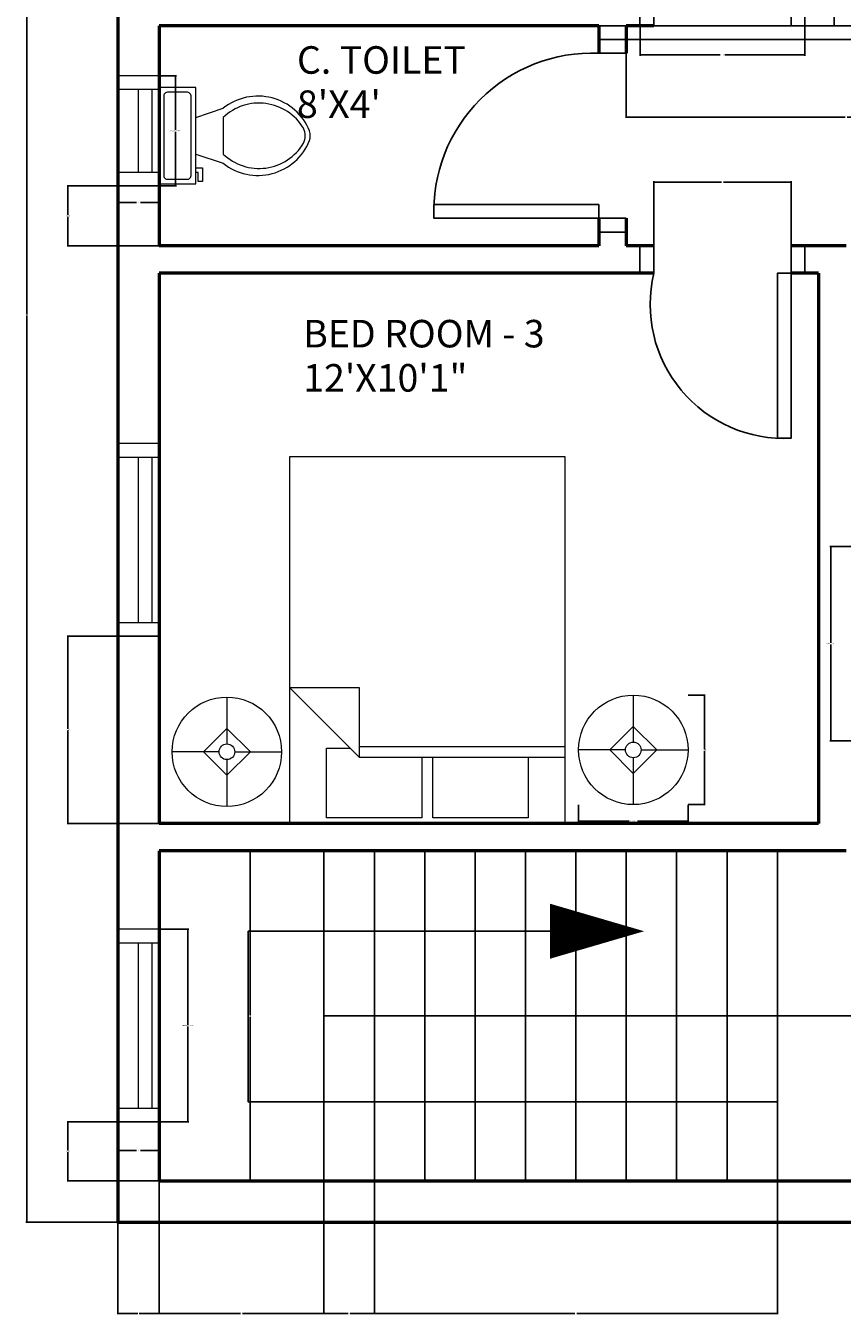
# Model space of a CAD drawing. Units: inches. Extents: x 2630 to 2982, y 643 to 1079.
# Tile 1 of 4: x 2630 to 2808, y 643 to 924. Entities that reach past the tile are written whole.
import ezdxf

# ---------------------------------------------------------------- set-up
doc = ezdxf.new("R2010")
doc.units = ezdxf.units.IN
for name, color, linetype, lineweight in [('A-ANNO-DIMS', 2, 'Continuous', 18), ('A-AREA-IDEN', 7, 'Continuous', 25), ('A-DOOR', 3, 'Continuous', 25), ('A-FLOR-FIXT', 9, 'Continuous', 18), ('A-FLOR-STRS', 7, 'Continuous', 25), ('A-FURN', 8, 'Continuous', 18), ('A-GLAZ', 4, 'Continuous', 18), ('A-WALL', 7, 'Continuous', 50)]:
    doc.layers.add(name, color=color, linetype=linetype, lineweight=lineweight)
doc.styles.get("Standard").update_dxf_attribs({"font": 'arial.ttf'})
doc.dimstyles.get("Standard").update_dxf_attribs({"dimtxt": 0.18, "dimasz": 0.18, "dimexe": 0.18, "dimexo": 0.0625, "dimgap": 0.09, "dimtad": 0, "dimtih": 1, "dimtoh": 1, "dimdec": 4, "dimzin": 0, "dimdsep": 46, "dimtxsty": 'Standard', "dimcen": 0.09, "dimadec": 0, "dimazin": 0, "dimtfac": 1, "dimtdec": 4, "dimtofl": 0, "dimtmove": 0, "dimatfit": 3, "dimfxl": 1, "dimtolj": 1, "dimtzin": 0, "dimarcsym": 0})

# ---------------------------------------------------------------- blocks, each defined once
blk = doc.blocks.new('Bed - Queen')
for p, q in [((0, -80.00003), (0, 0)), ((0, 0), (59.99999, 0)), ((59.99999, 0), (59.99999, -80.00003)), ((7.99999, -1.2), (28.79998, -1.2)), ((7.99999, -14.4), (7.99999, -1.2)), ((28.79998, -1.2), (28.79998, -14.4)), ((31.19999, -1.2), (51.99999, -1.2)), ((31.19999, -14.4), (31.19999, -1.2)), ((51.99999, -1.2), (51.99999, -16.4)), ((0, -14.4), (44.8, -14.4)), ((44.8, -16.8), (0, -16.8)), ((59.99999, -29.6), (44.8, -14.4)), ((44.8, -14.4), (44.8, -29.6)), ((51.99999, -16.4), (46.79936, -16.4)), ((44.8, -29.6), (59.99999, -29.6)), ((59.99999, -80.00003), (0, -80.00003))]:
    blk.add_line(p, q)
blk = doc.blocks.new('Lamp - Table')
for p, q in [((0, 7), (0, 1)), ((0, 3), (-3, 0)), ((3, 0), (0, 3)), ((-1, 0), (-7, 0)), ((-3, 0), (0, -3)), ((0, -3), (3, 0)), ((1, 0), (7, 0)), ((0, -1), (0, -7))]:
    blk.add_line(p, q)
for radius in [7, 1]:
    blk.add_circle((0, 0), radius)
blk = doc.blocks.new('Toilet - top')
for p, q in [((9.5, -6), (9.5, -2)), ((-8, -8.5), (-8, -8)), ((-7, -8), (-7, -9.5)), ((-4, -8), (-6, -14)), ((4, -8), (6, -14)), ((-10, -8.5), (-8, -8.5)), ((-10, -9.5), (-10, -8.5)), ((-7, -9.5), (-10, -9.5)), ((4, -14), (-4, -14))]:
    blk.add_line(p, q)
blk.add_lwpolyline([(10.5, -8), (10.5, 0), (-10.5, 0), (-10.5, -8)], close=True)
for points in [[(-9.5, -2), (-9.5, -6)], [(8.5, -1), (-8.5, -1)], [(-8.5, -7), (8.5, -7)]]:
    blk.add_lwpolyline(points)
for centre, radius, start, end in [((-8.62, -1.88), 0.884, 81.8699, 188.1301), ((8.62, -1.88), 0.884, 351.8699, 98.1301), ((-8.62, -6.12), 0.884, 171.8699, 278.1301), ((8.62, -6.12), 0.884, 261.8699, 8.1301), ((3.52, -21.58), 12.17, 141.4691, 247.9714), ((4.2, -21.82), 11.33, 136.3677, 238.9468), ((-3.52, -21.58), 12.17, 292.0284, 38.5307), ((-4.2, -21.82), 11.33, 301.053, 43.6321), ((0, -27.88), 4, 245.7318, 294.2682), ((0, -29), 4, 254.8605, 285.1395)]:
    blk.add_arc(centre, radius, start, end)
blk = doc.blocks.new('DOOR-30IN-INT')
for p, q in [((0, 6), (0, 0)), ((3, 6), (3, 0)), ((33, 6), (33, 0)), ((36, 6), (36, 0))]:
    blk.add_line(p, q)
blk.add_lwpolyline([(33, 6), (30, 6), (30, 42), (33, 42)], close=True)
blk.add_arc((31.5, 12.75), 29.29, 87.0643, 193.3245)
blk = doc.blocks.new('DOOR-36IN-INT')
for p, q in [((0, 6), (0, 0)), ((3, 6), (3, 0)), ((39, 6), (39, 0)), ((42, 6), (42, 0))]:
    blk.add_line(p, q)
blk.add_lwpolyline([(3, 6), (6, 6), (6, 42), (3, 42)], close=True)
blk.add_arc((4.5, 7.5), 34.53, 357.5104, 92.4896)
blk = doc.blocks.new('WIN-36IN')
for p, q in [((9, 42), (0, 42)), ((9, 39), (0, 39)), ((4.5, 3), (4.5, 39)), ((7.5, 3), (7.5, 39)), ((0, 3), (9, 3)), ((0, 0), (9, 0))]:
    blk.add_line(p, q)
blk = doc.blocks.new('WIN-18IN')
for p, q in [((9, 24), (0, 24)), ((9, 21), (0, 21)), ((1.5, 21), (1.5, 3)), ((4.5, 21), (4.5, 3)), ((0, 3), (9, 3)), ((0, 0), (9, 0))]:
    blk.add_line(p, q)
blk = doc.blocks.new('*D13')
at = {"layer": 'A-ANNO-DIMS', "color": 0, "lineweight": -2, "transparency": 16777216}
for p, q in [((2750.36, 753.89), (2750.36, 750.19)), ((2774.25, 753.89), (2774.25, 750.19)), ((2750.54, 750.37), (2761.41, 750.37)), ((2774.07, 750.37), (2763.21, 750.37))]:
    blk.add_line(p, q, dxfattribs=at)
at = {"layer": 'A-ANNO-DIMS', "color": 0, "transparency": 16777216}
for points in [[(2750.54, 750.4), (2750.54, 750.34), (2750.36, 750.37)], [(2774.07, 750.4), (2774.07, 750.34), (2774.25, 750.37)]]:
    blk.add_solid(points, dxfattribs=at)
at = {"layer": 'Defpoints', "color": 0, "transparency": 16777216}
for p in [(2750.36, 753.95), (2774.25, 753.95), (2774.25, 750.37)]:
    blk.add_point(p, dxfattribs=at)
at = {"layer": 'A-ANNO-DIMS', "color": 0, "transparency": 16777216, "insert": (2762.31, 750.37), "char_height": 0.18, "attachment_point": 5}
blk.add_mtext('\\A1;LAMP 24 TYP.', dxfattribs=at)
blk = doc.blocks.new('*D14')
at = {"layer": 'A-ANNO-DIMS', "color": 0, "lineweight": -2, "transparency": 16777216}
for p, q in [((2774.32, 777.84), (2778.02, 777.84)), ((2777.84, 777.66), (2777.84, 766.08)), ((2777.84, 754.13), (2777.84, 765.72)), ((2774.32, 753.95), (2778.02, 753.95))]:
    blk.add_line(p, q, dxfattribs=at)
at = {"layer": 'A-ANNO-DIMS', "color": 0, "transparency": 16777216}
for points in [[(2777.81, 777.66), (2777.87, 777.66), (2777.84, 777.84)], [(2777.81, 754.13), (2777.87, 754.13), (2777.84, 753.95)]]:
    blk.add_solid(points, dxfattribs=at)
at = {"layer": 'Defpoints', "color": 0, "transparency": 16777216}
for p in [(2774.25, 777.84), (2777.84, 777.84), (2774.25, 753.95)]:
    blk.add_point(p, dxfattribs=at)
at = {"layer": 'A-ANNO-DIMS', "color": 0, "transparency": 16777216, "insert": (2777.84, 765.9), "char_height": 0.18, "attachment_point": 5}
blk.add_mtext('\\A1;24 TYP.', dxfattribs=at)
blk = doc.blocks.new('*D15')
at = {"layer": 'A-ANNO-DIMS', "color": 0, "lineweight": -2, "transparency": 16777216}
for p, q in [((2658.83, 726.76), (2665.25, 726.76)), ((2665.07, 726.58), (2665.07, 705.94)), ((2665.07, 684.94), (2665.07, 705.58)), ((2658.83, 684.76), (2665.25, 684.76))]:
    blk.add_line(p, q, dxfattribs=at)
at = {"layer": 'A-ANNO-DIMS', "color": 0, "transparency": 16777216}
for points in [[(2665.04, 726.58), (2665.1, 726.58), (2665.07, 726.76)], [(2665.04, 684.94), (2665.1, 684.94), (2665.07, 684.76)]]:
    blk.add_solid(points, dxfattribs=at)
at = {"layer": 'Defpoints', "color": 0, "transparency": 16777216}
for p in [(2658.77, 726.76), (2665.07, 726.76), (2658.77, 684.76)]:
    blk.add_point(p, dxfattribs=at)
at = {"layer": 'A-ANNO-DIMS', "color": 0, "transparency": 16777216, "insert": (2665.07, 705.76), "char_height": 0.18, "attachment_point": 5}
blk.add_mtext('\\A1;WINDOW W1 42 TYP.', dxfattribs=at)
blk = doc.blocks.new('*D16')
at = {"layer": 'A-ANNO-DIMS', "color": 0, "lineweight": -2, "transparency": 16777216}
for p, q in [((2649.77, 684.7), (2649.77, 678.28)), ((2658.77, 684.7), (2658.77, 678.28)), ((2649.95, 678.46), (2653.81, 678.46)), ((2658.59, 678.46), (2654.73, 678.46))]:
    blk.add_line(p, q, dxfattribs=at)
at = {"layer": 'A-ANNO-DIMS', "color": 0, "transparency": 16777216}
for points in [[(2649.95, 678.49), (2649.95, 678.43), (2649.77, 678.46)], [(2658.59, 678.49), (2658.59, 678.43), (2658.77, 678.46)]]:
    blk.add_solid(points, dxfattribs=at)
at = {"layer": 'Defpoints', "color": 0, "transparency": 16777216}
for p in [(2649.77, 684.76), (2658.77, 684.76), (2658.77, 678.46)]:
    blk.add_point(p, dxfattribs=at)
at = {"layer": 'A-ANNO-DIMS', "color": 0, "transparency": 16777216, "insert": (2654.27, 678.46), "char_height": 0.18, "attachment_point": 5}
blk.add_mtext('\\A1;9 TYP.', dxfattribs=at)
blk = doc.blocks.new('*D19')
at = {"layer": 'A-ANNO-DIMS', "color": 0, "lineweight": -2, "transparency": 16777216}
for p, q in [((2811.7, 810.29), (2805.22, 810.29)), ((2805.4, 810.11), (2805.4, 789.26)), ((2805.4, 768.05), (2805.4, 788.89)), ((2811.7, 767.87), (2805.22, 767.87))]:
    blk.add_line(p, q, dxfattribs=at)
at = {"layer": 'A-ANNO-DIMS', "color": 0, "transparency": 16777216}
for points in [[(2805.37, 810.11), (2805.43, 810.11), (2805.4, 810.29)], [(2805.37, 768.05), (2805.43, 768.05), (2805.4, 767.87)]]:
    blk.add_solid(points, dxfattribs=at)
at = {"layer": 'Defpoints', "color": 0, "transparency": 16777216}
for p in [(2805.4, 810.29), (2811.77, 810.29), (2811.77, 767.87)]:
    blk.add_point(p, dxfattribs=at)
at = {"layer": 'A-ANNO-DIMS', "color": 0, "transparency": 16777216, "insert": (2805.4, 789.08), "char_height": 0.18, "attachment_point": 5}
blk.add_mtext('\\A1;DOOR D1 42 TYP.', dxfattribs=at)
blk = doc.blocks.new('*D25')
at = {"layer": 'A-ANNO-DIMS', "color": 0, "lineweight": -2, "transparency": 16777216}
for p, q in [((2799.83, 966.34), (2806.32, 966.34)), ((2806.14, 966.16), (2806.14, 945.29)), ((2806.14, 924.05), (2806.14, 944.92)), ((2799.83, 923.87), (2806.32, 923.87))]:
    blk.add_line(p, q, dxfattribs=at)
at = {"layer": 'A-ANNO-DIMS', "color": 0, "transparency": 16777216}
for points in [[(2806.11, 966.16), (2806.17, 966.16), (2806.14, 966.34)], [(2806.11, 924.05), (2806.17, 924.05), (2806.14, 923.87)]]:
    blk.add_solid(points, dxfattribs=at)
at = {"layer": 'Defpoints', "color": 0, "transparency": 16777216}
for p in [(2799.77, 966.34), (2806.14, 966.34), (2799.77, 923.87)]:
    blk.add_point(p, dxfattribs=at)
at = {"layer": 'A-ANNO-DIMS', "color": 0, "transparency": 16777216, "insert": (2806.14, 945.1), "char_height": 0.18, "attachment_point": 5}
blk.add_mtext('\\A1;DOOR D2 42 TYP.', dxfattribs=at)
blk = doc.blocks.new('*D26')
at = {"layer": 'A-ANNO-DIMS', "color": 0, "lineweight": -2, "transparency": 16777216}
for p, q in [((2763.77, 923.8), (2763.77, 917.32)), ((2799.77, 923.8), (2799.77, 917.32)), ((2763.95, 917.5), (2781.24, 917.5)), ((2799.59, 917.5), (2782.3, 917.5))]:
    blk.add_line(p, q, dxfattribs=at)
at = {"layer": 'A-ANNO-DIMS', "color": 0, "transparency": 16777216}
for points in [[(2763.95, 917.53), (2763.95, 917.47), (2763.77, 917.5)], [(2799.59, 917.53), (2799.59, 917.47), (2799.77, 917.5)]]:
    blk.add_solid(points, dxfattribs=at)
at = {"layer": 'Defpoints', "color": 0, "transparency": 16777216}
for p in [(2763.77, 923.87), (2799.77, 923.87), (2799.77, 917.5)]:
    blk.add_point(p, dxfattribs=at)
at = {"layer": 'A-ANNO-DIMS', "color": 0, "transparency": 16777216, "insert": (2781.77, 917.5), "char_height": 0.18, "attachment_point": 5}
blk.add_mtext('\\A1;36 TYP.', dxfattribs=at)
blk = doc.blocks.new('*D27')
at = {"layer": 'A-ANNO-DIMS', "color": 0, "lineweight": -2, "transparency": 16777216}
for p, q in [((2658.83, 912.94), (2662.55, 912.94)), ((2662.37, 912.76), (2662.37, 901.13)), ((2662.37, 889.12), (2662.37, 900.76)), ((2658.83, 888.94), (2662.55, 888.94))]:
    blk.add_line(p, q, dxfattribs=at)
at = {"layer": 'A-ANNO-DIMS', "color": 0, "transparency": 16777216}
for points in [[(2662.34, 912.76), (2662.4, 912.76), (2662.37, 912.94)], [(2662.34, 889.12), (2662.4, 889.12), (2662.37, 888.94)]]:
    blk.add_solid(points, dxfattribs=at)
at = {"layer": 'Defpoints', "color": 0, "transparency": 16777216}
for p in [(2658.77, 912.94), (2658.77, 888.94), (2662.37, 888.94)]:
    blk.add_point(p, dxfattribs=at)
at = {"layer": 'A-ANNO-DIMS', "color": 0, "transparency": 16777216, "insert": (2662.37, 900.94), "char_height": 0.18, "attachment_point": 5}
blk.add_mtext('\\A1;WINDOW W2 24 TYP.', dxfattribs=at)
blk = doc.blocks.new('*D28')
at = {"layer": 'A-ANNO-DIMS', "color": 0, "lineweight": -2, "transparency": 16777216}
for p, q in [((2649.77, 888.88), (2649.77, 885.16)), ((2658.77, 888.88), (2658.77, 885.16)), ((2649.95, 885.34), (2653.81, 885.34)), ((2658.59, 885.34), (2654.73, 885.34))]:
    blk.add_line(p, q, dxfattribs=at)
at = {"layer": 'A-ANNO-DIMS', "color": 0, "transparency": 16777216}
for points in [[(2649.95, 885.37), (2649.95, 885.31), (2649.77, 885.34)], [(2658.59, 885.37), (2658.59, 885.31), (2658.77, 885.34)]]:
    blk.add_solid(points, dxfattribs=at)
at = {"layer": 'Defpoints', "color": 0, "transparency": 16777216}
for p in [(2649.77, 888.94), (2658.77, 888.94), (2649.77, 885.34)]:
    blk.add_point(p, dxfattribs=at)
at = {"layer": 'A-ANNO-DIMS', "color": 0, "transparency": 16777216, "insert": (2654.27, 885.34), "char_height": 0.18, "attachment_point": 5}
blk.add_mtext('\\A1;9 TYP.', dxfattribs=at)
blk = doc.blocks.new('*D38')
at = {"layer": 'A-ANNO-DIMS', "color": 0, "lineweight": -2, "transparency": 16777216}
for p, q in [((2649.7, 1058.87), (2629.68, 1058.87)), ((2629.86, 1058.69), (2629.86, 861.05)), ((2629.86, 663.05), (2629.86, 860.68)), ((2649.7, 662.87), (2629.68, 662.87))]:
    blk.add_line(p, q, dxfattribs=at)
at = {"layer": 'A-ANNO-DIMS', "color": 0, "transparency": 16777216}
for points in [[(2629.83, 1058.69), (2629.89, 1058.69), (2629.86, 1058.87)], [(2629.83, 663.05), (2629.89, 663.05), (2629.86, 662.87)]]:
    blk.add_solid(points, dxfattribs=at)
at = {"layer": 'Defpoints', "color": 0, "transparency": 16777216}
for p in [(2629.86, 1058.87), (2649.77, 1058.87), (2649.77, 662.87)]:
    blk.add_point(p, dxfattribs=at)
at = {"layer": 'A-ANNO-DIMS', "color": 0, "transparency": 16777216, "insert": (2629.86, 860.87), "char_height": 0.18, "attachment_point": 5}
blk.add_mtext('\\A1;396', dxfattribs=at)
blk = doc.blocks.new('*D39')
at = {"layer": 'A-ANNO-DIMS', "color": 0, "lineweight": -2, "transparency": 16777216}
for p, q in [((2658.77, 671.8), (2658.77, 642.78)), ((2649.77, 662.8), (2649.77, 642.78)), ((2649.95, 642.96), (2654.12, 642.96)), ((2658.59, 642.96), (2654.42, 642.96))]:
    blk.add_line(p, q, dxfattribs=at)
at = {"layer": 'A-ANNO-DIMS', "color": 0, "transparency": 16777216}
for points in [[(2649.95, 642.99), (2649.95, 642.93), (2649.77, 642.96)], [(2658.59, 642.99), (2658.59, 642.93), (2658.77, 642.96)]]:
    blk.add_solid(points, dxfattribs=at)
at = {"layer": 'Defpoints', "color": 0, "transparency": 16777216}
for p in [(2658.77, 671.87), (2649.77, 662.87), (2658.77, 642.96)]:
    blk.add_point(p, dxfattribs=at)
at = {"layer": 'A-ANNO-DIMS', "color": 0, "transparency": 16777216, "insert": (2654.27, 642.96), "char_height": 0.18, "attachment_point": 5}
blk.add_mtext('\\A1;9', dxfattribs=at)
blk = doc.blocks.new('*D42')
at = {"layer": 'A-ANNO-DIMS', "color": 0, "lineweight": -2, "transparency": 16777216}
for p, q in [((2658.7, 888.94), (2638.68, 888.94)), ((2638.86, 888.76), (2638.86, 882.59)), ((2638.86, 876.05), (2638.86, 882.22)), ((2658.7, 875.87), (2638.68, 875.87))]:
    blk.add_line(p, q, dxfattribs=at)
at = {"layer": 'A-ANNO-DIMS', "color": 0, "transparency": 16777216}
for points in [[(2638.83, 888.76), (2638.89, 888.76), (2638.86, 888.94)], [(2638.83, 876.05), (2638.89, 876.05), (2638.86, 875.87)]]:
    blk.add_solid(points, dxfattribs=at)
at = {"layer": 'Defpoints', "color": 0, "transparency": 16777216}
for p in [(2638.86, 888.94), (2658.77, 888.94), (2658.77, 875.87)]:
    blk.add_point(p, dxfattribs=at)
at = {"layer": 'A-ANNO-DIMS', "color": 0, "transparency": 16777216, "insert": (2638.86, 882.41), "char_height": 0.18, "attachment_point": 5}
blk.add_mtext('\\A1;13.078', dxfattribs=at)
blk = doc.blocks.new('*D43')
at = {"layer": 'A-ANNO-DIMS', "color": 0, "lineweight": -2, "transparency": 16777216}
for p, q in [((2658.7, 790.7), (2638.68, 790.7)), ((2638.86, 790.52), (2638.86, 770.47)), ((2638.86, 750.05), (2638.86, 770.1)), ((2658.7, 749.87), (2638.68, 749.87))]:
    blk.add_line(p, q, dxfattribs=at)
at = {"layer": 'A-ANNO-DIMS', "color": 0, "transparency": 16777216}
for points in [[(2638.83, 790.52), (2638.89, 790.52), (2638.86, 790.7)], [(2638.83, 750.05), (2638.89, 750.05), (2638.86, 749.87)]]:
    blk.add_solid(points, dxfattribs=at)
at = {"layer": 'Defpoints', "color": 0, "transparency": 16777216}
for p in [(2638.86, 790.7), (2658.77, 790.7), (2658.77, 749.87)]:
    blk.add_point(p, dxfattribs=at)
at = {"layer": 'A-ANNO-DIMS', "color": 0, "transparency": 16777216, "insert": (2638.86, 770.28), "char_height": 0.18, "attachment_point": 5}
blk.add_mtext('\\A1;40.83', dxfattribs=at)
blk = doc.blocks.new('*D44')
at = {"layer": 'A-ANNO-DIMS', "color": 0, "lineweight": -2, "transparency": 16777216}
for p, q in [((2658.7, 684.76), (2638.68, 684.76)), ((2638.86, 684.58), (2638.86, 678.5)), ((2638.86, 672.05), (2638.86, 678.13)), ((2658.7, 671.87), (2638.68, 671.87))]:
    blk.add_line(p, q, dxfattribs=at)
at = {"layer": 'A-ANNO-DIMS', "color": 0, "transparency": 16777216}
for points in [[(2638.83, 684.58), (2638.89, 684.58), (2638.86, 684.76)], [(2638.83, 672.05), (2638.89, 672.05), (2638.86, 671.87)]]:
    blk.add_solid(points, dxfattribs=at)
at = {"layer": 'Defpoints', "color": 0, "transparency": 16777216}
for p in [(2638.86, 684.76), (2658.77, 684.76), (2658.77, 671.87)]:
    blk.add_point(p, dxfattribs=at)
at = {"layer": 'A-ANNO-DIMS', "color": 0, "transparency": 16777216, "insert": (2638.86, 678.31), "char_height": 0.18, "attachment_point": 5}
blk.add_mtext('\\A1;12.894', dxfattribs=at)
blk = doc.blocks.new('*D53')
at = {"layer": 'A-ANNO-DIMS', "color": 0, "lineweight": -2, "transparency": 16777216}
for p, q in [((2793.83, 707.87), (2813.86, 707.87)), ((2813.68, 707.69), (2813.68, 690.05)), ((2813.68, 672.05), (2813.68, 689.68)), ((2793.83, 671.87), (2813.86, 671.87))]:
    blk.add_line(p, q, dxfattribs=at)
at = {"layer": 'A-ANNO-DIMS', "color": 0, "transparency": 16777216}
for points in [[(2813.65, 707.69), (2813.71, 707.69), (2813.68, 707.87)], [(2813.65, 672.05), (2813.71, 672.05), (2813.68, 671.87)]]:
    blk.add_solid(points, dxfattribs=at)
at = {"layer": 'Defpoints', "color": 0, "transparency": 16777216}
for p in [(2793.77, 707.87), (2793.77, 671.87), (2813.68, 671.87)]:
    blk.add_point(p, dxfattribs=at)
at = {"layer": 'A-ANNO-DIMS', "color": 0, "transparency": 16777216, "insert": (2813.68, 689.87), "char_height": 0.18, "attachment_point": 5}
blk.add_mtext('\\A1;36', dxfattribs=at)
blk = doc.blocks.new('*D54')
at = {"layer": 'A-ANNO-DIMS', "color": 0, "lineweight": -2, "transparency": 16777216}
for p, q in [((2658.77, 671.8), (2658.77, 642.78)), ((2694.77, 671.8), (2694.77, 642.78)), ((2658.95, 642.96), (2676.55, 642.96)), ((2694.59, 642.96), (2676.99, 642.96))]:
    blk.add_line(p, q, dxfattribs=at)
at = {"layer": 'A-ANNO-DIMS', "color": 0, "transparency": 16777216}
for points in [[(2658.95, 642.99), (2658.95, 642.93), (2658.77, 642.96)], [(2694.59, 642.99), (2694.59, 642.93), (2694.77, 642.96)]]:
    blk.add_solid(points, dxfattribs=at)
at = {"layer": 'Defpoints', "color": 0, "transparency": 16777216}
for p in [(2658.77, 671.87), (2694.77, 671.87), (2694.77, 642.96)]:
    blk.add_point(p, dxfattribs=at)
at = {"layer": 'A-ANNO-DIMS', "color": 0, "transparency": 16777216, "insert": (2676.77, 642.96), "char_height": 0.18, "attachment_point": 5}
blk.add_mtext('\\A1;36', dxfattribs=at)
blk = doc.blocks.new('*D55')
at = {"layer": 'A-ANNO-DIMS', "color": 0, "lineweight": -2, "transparency": 16777216}
for p, q in [((2694.77, 671.8), (2694.77, 642.78)), ((2705.77, 671.8), (2705.77, 642.78)), ((2694.95, 642.96), (2700.07, 642.96)), ((2705.59, 642.96), (2700.46, 642.96))]:
    blk.add_line(p, q, dxfattribs=at)
at = {"layer": 'A-ANNO-DIMS', "color": 0, "transparency": 16777216}
for points in [[(2694.95, 642.99), (2694.95, 642.93), (2694.77, 642.96)], [(2705.59, 642.99), (2705.59, 642.93), (2705.77, 642.96)]]:
    blk.add_solid(points, dxfattribs=at)
at = {"layer": 'Defpoints', "color": 0, "transparency": 16777216}
for p in [(2694.77, 671.87), (2705.77, 671.87), (2705.77, 642.96)]:
    blk.add_point(p, dxfattribs=at)
at = {"layer": 'A-ANNO-DIMS', "color": 0, "transparency": 16777216, "insert": (2700.27, 642.96), "char_height": 0.18, "attachment_point": 5}
blk.add_mtext('\\A1;11', dxfattribs=at)
blk = doc.blocks.new('*D56')
at = {"layer": 'A-ANNO-DIMS', "color": 0, "lineweight": -2, "transparency": 16777216}
for p, q in [((2705.77, 671.8), (2705.77, 642.78)), ((2793.77, 671.8), (2793.77, 642.78)), ((2705.95, 642.96), (2749.55, 642.96)), ((2793.59, 642.96), (2749.99, 642.96))]:
    blk.add_line(p, q, dxfattribs=at)
at = {"layer": 'A-ANNO-DIMS', "color": 0, "transparency": 16777216}
for points in [[(2705.95, 642.99), (2705.95, 642.93), (2705.77, 642.96)], [(2793.59, 642.99), (2793.59, 642.93), (2793.77, 642.96)]]:
    blk.add_solid(points, dxfattribs=at)
at = {"layer": 'Defpoints', "color": 0, "transparency": 16777216}
for p in [(2705.77, 671.87), (2793.77, 671.87), (2793.77, 642.96)]:
    blk.add_point(p, dxfattribs=at)
at = {"layer": 'A-ANNO-DIMS', "color": 0, "transparency": 16777216, "insert": (2749.77, 642.96), "char_height": 0.18, "attachment_point": 5}
blk.add_mtext('\\A1;88', dxfattribs=at)
blk = doc.blocks.new('*D61')
at = {"layer": 'A-ANNO-DIMS', "color": 0, "lineweight": -2, "transparency": 16777216}
for p, q in [((2754.83, 923.87), (2981.86, 923.87)), ((2981.68, 923.69), (2981.68, 922.55)), ((2981.68, 921.05), (2981.68, 922.18)), ((2754.83, 920.87), (2981.86, 920.87))]:
    blk.add_line(p, q, dxfattribs=at)
at = {"layer": 'A-ANNO-DIMS', "color": 0, "transparency": 16777216}
for points in [[(2981.65, 923.69), (2981.71, 923.69), (2981.68, 923.87)], [(2981.65, 921.05), (2981.71, 921.05), (2981.68, 920.87)]]:
    blk.add_solid(points, dxfattribs=at)
at = {"layer": 'Defpoints', "color": 0, "transparency": 16777216}
for p in [(2754.77, 923.87), (2754.77, 920.87), (2981.68, 920.87)]:
    blk.add_point(p, dxfattribs=at)
at = {"layer": 'A-ANNO-DIMS', "color": 0, "transparency": 16777216, "insert": (2981.68, 922.37), "char_height": 0.18, "attachment_point": 5}
blk.add_mtext('\\A1;3', dxfattribs=at)
blk = doc.blocks.new('*D62')
at = {"layer": 'A-ANNO-DIMS', "color": 0, "lineweight": -2, "transparency": 16777216}
for p, q in [((2766.77, 869.93), (2766.77, 889.96)), ((2766.95, 889.78), (2781.55, 889.78)), ((2796.59, 889.78), (2781.99, 889.78)), ((2796.77, 869.93), (2796.77, 889.96))]:
    blk.add_line(p, q, dxfattribs=at)
at = {"layer": 'A-ANNO-DIMS', "color": 0, "transparency": 16777216}
for points in [[(2766.95, 889.81), (2766.95, 889.75), (2766.77, 889.78)], [(2796.59, 889.81), (2796.59, 889.75), (2796.77, 889.78)]]:
    blk.add_solid(points, dxfattribs=at)
at = {"layer": 'Defpoints', "color": 0, "transparency": 16777216}
for p in [(2796.77, 889.78), (2766.77, 869.87), (2796.77, 869.87)]:
    blk.add_point(p, dxfattribs=at)
at = {"layer": 'A-ANNO-DIMS', "color": 0, "transparency": 16777216, "insert": (2781.77, 889.78), "char_height": 0.18, "attachment_point": 5}
blk.add_mtext('\\A1;30', dxfattribs=at)
blk = doc.blocks.new('*D64')
at = {"layer": 'A-ANNO-DIMS', "color": 0, "lineweight": -2, "transparency": 16777216}
for p, q in [((2760.77, 923.8), (2760.77, 903.78)), ((2856.77, 923.8), (2856.77, 903.78)), ((2760.95, 903.96), (2808.55, 903.96)), ((2856.59, 903.96), (2808.99, 903.96))]:
    blk.add_line(p, q, dxfattribs=at)
at = {"layer": 'A-ANNO-DIMS', "color": 0, "transparency": 16777216}
for points in [[(2760.95, 903.99), (2760.95, 903.93), (2760.77, 903.96)], [(2856.59, 903.99), (2856.59, 903.93), (2856.77, 903.96)]]:
    blk.add_solid(points, dxfattribs=at)
at = {"layer": 'Defpoints', "color": 0, "transparency": 16777216}
for p in [(2760.77, 923.87), (2856.77, 923.87), (2760.77, 903.96)]:
    blk.add_point(p, dxfattribs=at)
at = {"layer": 'A-ANNO-DIMS', "color": 0, "transparency": 16777216, "insert": (2808.77, 903.96), "char_height": 0.18, "attachment_point": 5}
blk.add_mtext('\\A1;96', dxfattribs=at)
blk = doc.blocks.new('*D65')
at = {"layer": 'A-ANNO-DIMS', "color": 0, "lineweight": -2, "transparency": 16777216}
for p, q in [((2658.83, 743.87), (2678.86, 743.87)), ((2678.68, 743.69), (2678.68, 708.05)), ((2678.68, 672.05), (2678.68, 707.69)), ((2658.83, 671.87), (2678.86, 671.87))]:
    blk.add_line(p, q, dxfattribs=at)
at = {"layer": 'A-ANNO-DIMS', "color": 0, "transparency": 16777216}
for points in [[(2678.65, 743.69), (2678.71, 743.69), (2678.68, 743.87)], [(2678.65, 672.05), (2678.71, 672.05), (2678.68, 671.87)]]:
    blk.add_solid(points, dxfattribs=at)
at = {"layer": 'Defpoints', "color": 0, "transparency": 16777216}
for p in [(2658.77, 743.87), (2658.77, 671.87), (2678.68, 671.87)]:
    blk.add_point(p, dxfattribs=at)
at = {"layer": 'A-ANNO-DIMS', "color": 0, "transparency": 16777216, "insert": (2678.68, 707.87), "char_height": 0.18, "attachment_point": 5}
blk.add_mtext('\\A1;72', dxfattribs=at)

msp = doc.modelspace()

# ---------------------------------------------------------------- linework, layer by layer
at = {"layer": 'A-FLOR-STRS'}
for p, q in [((2694.7671, 743.8666), (2694.7671, 671.8666)), ((2705.7671, 743.8666), (2705.7671, 671.8666)), ((2716.7671, 743.8666), (2716.7671, 671.8666)), ((2727.7671, 743.8666), (2727.7671, 671.8666)), ((2738.7671, 743.8666), (2738.7671, 671.8666)), ((2749.7671, 743.8666), (2749.7671, 671.8666)), ((2760.7671, 743.8666), (2760.7671, 671.8666)), ((2771.7671, 743.8666), (2771.7671, 671.8666)), ((2782.7671, 743.8666), (2782.7671, 671.8666)), ((2793.7671, 743.8666), (2793.7671, 671.8666)), ((2793.7671, 707.8666), (2694.7671, 707.8666))]:
    msp.add_line(p, q, dxfattribs=at)
msp.add_lwpolyline([(2744.1329, 726.3329, 12, 0, 0), (2764.6647, 726.3329, 0, 0, 0)], format="xyseb", dxfattribs=at)
msp.add_lwpolyline([(2793.7671, 689.0821), (2678.2153, 689.0821), (2678.2153, 726.3329), (2744.1329, 726.3329)], dxfattribs=at)
at = {"layer": 'A-WALL'}
for p, q in [((2658.7671, 923.8666), (2658.7671, 875.8666)), ((2754.7671, 923.8666), (2658.7671, 923.8666)), ((2754.7671, 923.8666), (2754.7671, 917.8666)), ((2760.7671, 923.8666), (2760.7671, 917.8666)), ((2766.7671, 923.8666), (2760.7671, 923.8666)), ((2754.7671, 881.8666), (2754.7671, 875.8666)), ((2760.7671, 881.8666), (2760.7671, 875.8666)), ((2754.7671, 875.8666), (2658.7671, 875.8666)), ((2766.7671, 875.8666), (2760.7671, 875.8666)), ((2808.7671, 875.8666), (2796.7671, 875.8666)), ((2658.7671, 869.8666), (2658.7671, 749.8666)), ((2766.7671, 869.8666), (2658.7671, 869.8666)), ((2802.7671, 869.8666), (2796.7671, 869.8666)), ((2802.7671, 869.8666), (2802.7671, 749.8666)), ((2802.7671, 749.8666), (2658.7671, 749.8666)), ((2808.7671, 743.8666), (2658.7671, 743.8666)), ((2658.7671, 743.8666), (2658.7671, 671.8666)), ((2658.7671, 671.8666), (2814.7671, 671.8666))]:
    msp.add_line(p, q, dxfattribs=at)
msp.add_lwpolyline([(2850.7671, 662.8666), (2961.7671, 662.8666), (2961.7671, 1058.8666), (2649.7671, 1058.8666), (2649.7671, 662.8666), (2814.7671, 662.8666)], dxfattribs=at)

# ---------------------------------------------------------------- block references
at = {"layer": 'A-DOOR'}
msp.add_blockref('DOOR-30IN-INT', (2763.767, 923.867), dxfattribs=at)
at = {"layer": 'A-DOOR', "rotation": 90.00000000000036}
msp.add_blockref('DOOR-36IN-INT', (2760.7667, 878.8665), dxfattribs=at)
at = {"layer": 'A-DOOR', "extrusion": (0, 0, -1), "zscale": -1, "rotation": 180}
msp.add_blockref('DOOR-30IN-INT', (-2763.767, 875.8663), dxfattribs=at)
at = {"layer": 'A-FLOR-FIXT', "rotation": 90}
msp.add_blockref('Toilet - top', (2658.7671, 899.8666), dxfattribs=at)
at = {"layer": 'A-FURN', "rotation": 180}
msp.add_blockref('Bed - Queen', (2747.3366, 749.8666), dxfattribs=at)
at = {"layer": 'A-FURN', "xscale": 1.706595897520738, "yscale": 1.706595897520738, "zscale": 1.706595897520738}
for p in [(2673.5711, 765.4739), (2762.3072, 765.8961)]:
    msp.add_blockref('Lamp - Table', p, dxfattribs=at)
at = {"layer": 'A-GLAZ', "rotation": 180}
msp.add_blockref('WIN-18IN', (2658.7672, 912.9445), dxfattribs=at)
at = {"layer": 'A-GLAZ'}
for p in [(2649.767, 790.6998), (2649.767, 684.7608)]:
    msp.add_blockref('WIN-36IN', p, dxfattribs=at)

# ---------------------------------------------------------------- texts
at = {"layer": 'A-AREA-IDEN'}
for s, p in [('C. TOILET', (2688.8661, 913.4037)), ("8'X4'", (2688.8661, 903.7653)), ('BED ROOM - 3', (2690.233, 853.6959)), ('12\'X10\'1"', (2690.233, 844.0574))]:
    msp.add_text(s, height=6, dxfattribs=at).set_placement(p)

# ---------------------------------------------------------------- dimensions: what is measured, and where the dimension line sits
at = {"layer": 'A-ANNO-DIMS'}
for base, p1, p2, angle, override, picture, middle in [((2629.8571, 1058.8666), (2649.7671, 662.8666), (2649.7671, 1058.8666), 90, {"dimdec": 0, "dimlfac": 1, "dimrnd": 0, "dimzin": 0, "dimdsep": 46, "dimlunit": 2}, '*D38', (2629.8571, 860.8666)), ((2981.6771, 920.8666), (2754.7671, 923.8666), (2754.7671, 920.8666), 90, {"dimdec": 0, "dimlfac": 1, "dimrnd": 0, "dimzin": 0, "dimdsep": 46, "dimlunit": 2}, '*D61', (2981.6771, 922.3666)), ((2760.7671, 903.9566), (2856.7671, 923.8666), (2760.7671, 923.8666), 180, {"dimdec": 0, "dimlfac": 1, "dimrnd": 0, "dimzin": 0, "dimdsep": 46, "dimlunit": 2}, '*D64', (2808.7671, 903.9566)), ((2638.8571, 888.9447), (2658.7671, 875.8666), (2658.7671, 888.9447), 90, {"dimdec": 3, "dimlfac": 1, "dimrnd": 0, "dimzin": 0, "dimdsep": 46, "dimlunit": 2}, '*D42', (2638.8571, 882.4057)), ((2638.8571, 790.6997), (2658.7671, 749.8666), (2658.7671, 790.6997), 90, {"dimdec": 2, "dimlfac": 1, "dimrnd": 0, "dimzin": 0, "dimdsep": 46, "dimlunit": 2}, '*D43', (2638.8571, 770.2832)), ((2678.6771, 671.8666), (2658.7671, 743.8666), (2658.7671, 671.8666), 270, {"dimdec": 0, "dimlfac": 1, "dimrnd": 0, "dimzin": 0, "dimdsep": 46, "dimlunit": 2}, '*D65', (2678.6771, 707.8666)), ((2813.6771, 671.8666), (2793.7671, 707.8666), (2793.7671, 671.8666), 270, {"dimdec": 0, "dimlfac": 1, "dimrnd": 0, "dimzin": 0, "dimdsep": 46, "dimlunit": 2}, '*D53', (2813.6771, 689.8666)), ((2638.8571, 684.7607), (2658.7671, 671.8666), (2658.7671, 684.7607), 90, {"dimdec": 3, "dimlfac": 1, "dimrnd": 0, "dimzin": 0, "dimdsep": 46, "dimlunit": 2}, '*D44', (2638.8571, 678.3137))]:
    dim = msp.add_linear_dim(base=base, p1=p1, p2=p2, angle=angle, dimstyle='Standard', override=override, dxfattribs=at)
    dim.commit()
    dim.dimension.update_dxf_attribs({"geometry": picture, "text_midpoint": middle})
for base, p1, p2, angle, text, picture, middle in [((2806.1379, 966.3388), (2799.7671, 923.8666), (2799.7671, 966.3388), 90, 'DOOR D2 <> TYP.', '*D25', (2806.1379, 945.1027)), ((2662.3671, 888.9447), (2658.7671, 912.9447), (2658.7671, 888.9447), 270, 'WINDOW W2 <> TYP.', '*D27', (2662.3671, 900.9447)), ((2649.7671, 885.3447), (2658.7671, 888.9447), (2649.7671, 888.9447), 180, '<> TYP.', '*D28', (2654.2671, 885.3447)), ((2805.404, 810.2871), (2811.7671, 767.8666), (2811.7671, 810.2871), 90, 'DOOR D1 <> TYP.', '*D19', (2805.404, 789.0769)), ((2777.8372, 777.8423), (2774.2534, 753.9499), (2774.2534, 777.8423), 90, '<> TYP.', '*D14', (2777.8372, 765.8961)), ((2665.0671, 726.7607), (2658.7671, 684.7607), (2658.7671, 726.7607), 90, 'WINDOW W1 <> TYP.', '*D15', (2665.0671, 705.7607))]:
    dim = msp.add_linear_dim(base=base, p1=p1, p2=p2, angle=angle, text=text, dimstyle='Standard', override={"dimdec": 0, "dimlfac": 1, "dimrnd": 0, "dimzin": 0, "dimdsep": 46, "dimlunit": 2}, dxfattribs=at)
    dim.commit()
    dim.dimension.update_dxf_attribs({"geometry": picture, "text_midpoint": middle})
for base, p1, p2, text, picture, middle in [((2799.7671, 917.4958), (2763.7671, 923.8666), (2799.7671, 923.8666), '<> TYP.', '*D26', (2781.7671, 917.4958)), ((2774.2534, 750.3661), (2750.361, 753.9499), (2774.2534, 753.9499), 'LAMP <> TYP.', '*D13', (2762.3072, 750.3661)), ((2658.7671, 678.4607), (2649.7671, 684.7607), (2658.7671, 684.7607), '<> TYP.', '*D16', (2654.2671, 678.4607))]:
    dim = msp.add_linear_dim(base=base, p1=p1, p2=p2, text=text, dimstyle='Standard', override={"dimdec": 0, "dimlfac": 1, "dimrnd": 0, "dimzin": 0, "dimdsep": 46, "dimlunit": 2}, dxfattribs=at)
    dim.commit()
    dim.dimension.update_dxf_attribs({"geometry": picture, "text_midpoint": middle})
for base, p1, p2, picture, middle in [((2796.7671, 889.7766), (2766.7671, 869.8666), (2796.7671, 869.8666), '*D62', (2781.7671, 889.7766)), ((2658.7671, 642.9566), (2649.7671, 662.8666), (2658.7671, 671.8666), '*D39', (2654.2671, 642.9566)), ((2694.7671, 642.9566), (2658.7671, 671.8666), (2694.7671, 671.8666), '*D54', (2676.7671, 642.9566)), ((2705.7671, 642.9566), (2694.7671, 671.8666), (2705.7671, 671.8666), '*D55', (2700.2671, 642.9566)), ((2793.7671, 642.9566), (2705.7671, 671.8666), (2793.7671, 671.8666), '*D56', (2749.7671, 642.9566))]:
    dim = msp.add_linear_dim(base=base, p1=p1, p2=p2, dimstyle='Standard', override={"dimdec": 0, "dimlfac": 1, "dimrnd": 0, "dimzin": 0, "dimdsep": 46, "dimlunit": 2}, dxfattribs=at)
    dim.commit()
    dim.dimension.update_dxf_attribs({"geometry": picture, "text_midpoint": middle})

doc.saveas('drawing.dxf')
